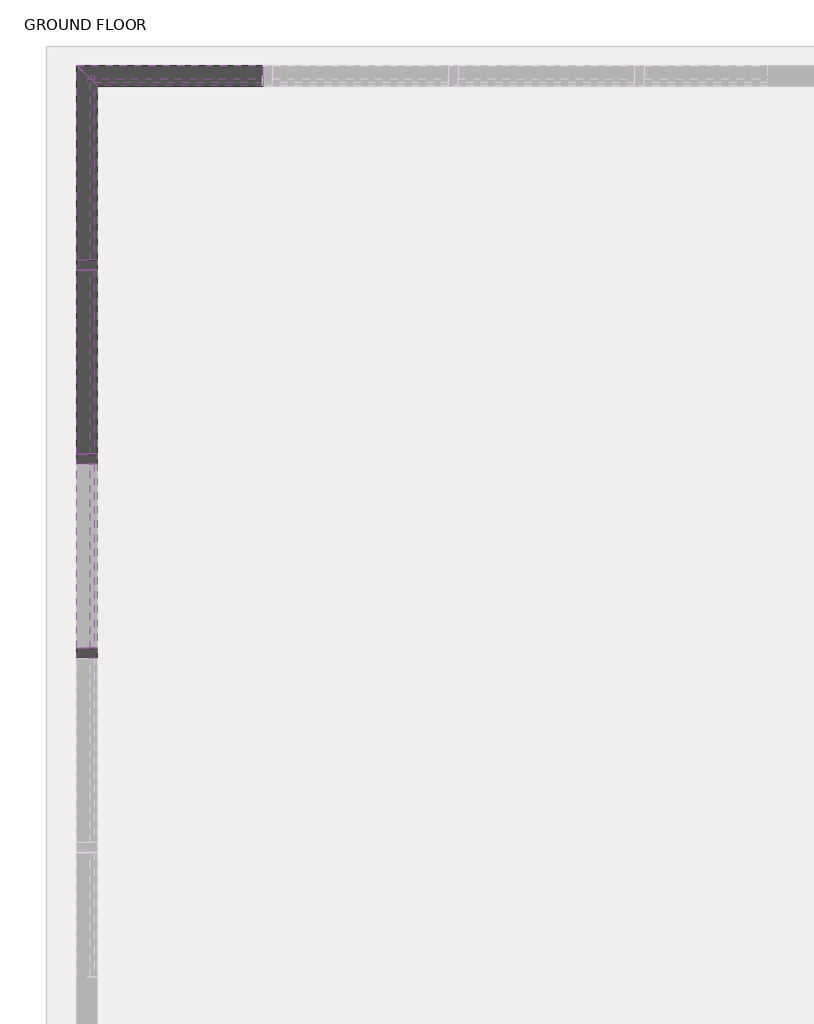
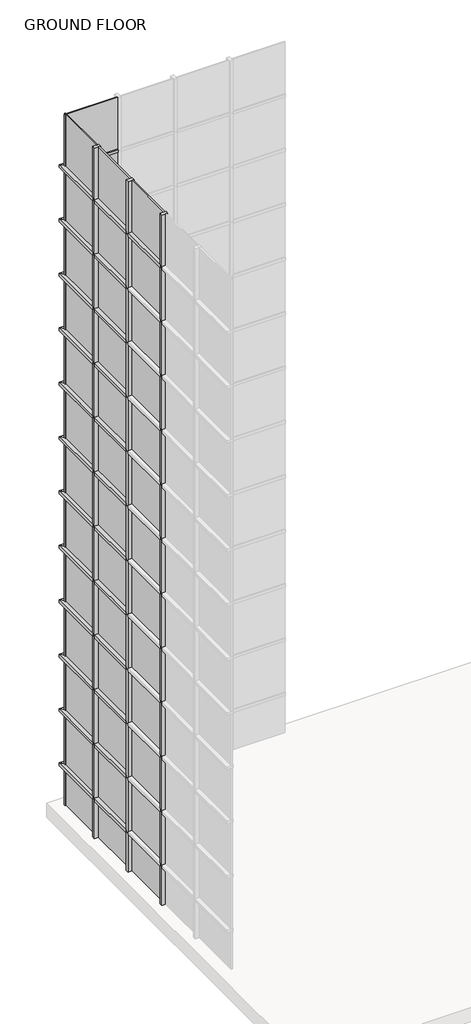
# One storey, part 8 of 16: 76 members, 53 plates.
"""IFC4 building model written with IfcOpenShell, lengths in millimetres."""

from ifc_helpers import new_model, si_unit, origin, place, context, project, spatial, transform, mapped, element, save
from components import member_80100a85, member_b860638c, member_31fee25f, member_49b1bc66, member_a361ce75, system_panel_glazed_5cba32e5, system_panel_glazed_49652e9e

model = new_model("IFC4")

# Units and contexts
model_context = context("Model", 3, world=origin())
ifc_project = project(units=[si_unit("LENGTHUNIT", "METRE", prefix="MILLI")], contexts=[model_context])

# Site, building, storey
site = spatial("IfcSite", under=ifc_project)
building = spatial("IfcBuilding", under=site)
storey = spatial("IfcBuildingStorey", under=building, Name="GROUND FLOOR", Elevation=0.0)

# Members
placement = place(None, origin())
member_shape = member_80100a85(model_context)
element("IfcMember", 1, ObjectType="Rectangular Mullion : 2.5\" x 5\" rectangular", at=placement, inside=storey, context=model_context, shape_type="MappedRepresentation", body=[
    mapped(member_shape, transform((-9124.9017534, 5216.4311965, 1168.8884615), x_axis=(0.0, 0.0, 1.0), y_axis=(-1.0, 0.0, 0.0), z_axis=(0.0, -1.0, 0.0))),
])
element("IfcMember", 2, ObjectType="Rectangular Mullion : 2.5\" x 5\" rectangular", at=placement, inside=storey, context=model_context, shape_type="MappedRepresentation", body=[
    mapped(member_shape, transform((-9124.9017534, 5216.4311965, 2369.5269231), x_axis=(0.0, 0.0, 1.0), y_axis=(-1.0, 0.0, 0.0), z_axis=(0.0, -1.0, 0.0))),
])
element("IfcMember", 3, ObjectType="Rectangular Mullion : 2.5\" x 5\" rectangular", at=placement, inside=storey, context=model_context, shape_type="MappedRepresentation", body=[
    mapped(member_shape, transform((-9124.9017534, 5216.4311965, 3570.1653846), x_axis=(0.0, 0.0, 1.0), y_axis=(-1.0, 0.0, 0.0), z_axis=(0.0, -1.0, 0.0))),
])
element("IfcMember", 4, ObjectType="Rectangular Mullion : 2.5\" x 5\" rectangular", at=placement, inside=storey, context=model_context, shape_type="MappedRepresentation", body=[
    mapped(member_shape, transform((-9124.9017534, 5216.4311965, 4770.8038462), x_axis=(0.0, 0.0, 1.0), y_axis=(-1.0, 0.0, 0.0), z_axis=(0.0, -1.0, 0.0))),
])
element("IfcMember", 5, ObjectType="Rectangular Mullion : 2.5\" x 5\" rectangular", at=placement, inside=storey, context=model_context, shape_type="MappedRepresentation", body=[
    mapped(member_shape, transform((-9124.9017534, 5216.4311965, 5971.4423077), x_axis=(0.0, 0.0, 1.0), y_axis=(-1.0, 0.0, 0.0), z_axis=(0.0, -1.0, 0.0))),
])
element("IfcMember", 6, ObjectType="Rectangular Mullion : 2.5\" x 5\" rectangular", at=placement, inside=storey, context=model_context, shape_type="MappedRepresentation", body=[
    mapped(member_shape, transform((-9124.9017534, 5216.4311965, 7172.0807692), x_axis=(0.0, 0.0, 1.0), y_axis=(-1.0, 0.0, 0.0), z_axis=(0.0, -1.0, 0.0))),
])
element("IfcMember", 7, ObjectType="Rectangular Mullion : 2.5\" x 5\" rectangular", at=placement, inside=storey, context=model_context, shape_type="MappedRepresentation", body=[
    mapped(member_shape, transform((-9124.9017534, 5216.4311965, 8372.7192308), x_axis=(0.0, 0.0, 1.0), y_axis=(-1.0, 0.0, 0.0), z_axis=(0.0, -1.0, 0.0))),
])
element("IfcMember", 8, ObjectType="Rectangular Mullion : 2.5\" x 5\" rectangular", at=placement, inside=storey, context=model_context, shape_type="MappedRepresentation", body=[
    mapped(member_shape, transform((-9124.9017534, 5216.4311965, 9573.3576923), x_axis=(0.0, 0.0, 1.0), y_axis=(-1.0, 0.0, 0.0), z_axis=(0.0, -1.0, 0.0))),
])
element("IfcMember", 9, ObjectType="Rectangular Mullion : 2.5\" x 5\" rectangular", at=placement, inside=storey, context=model_context, shape_type="MappedRepresentation", body=[
    mapped(member_shape, transform((-9124.9017534, 5216.4311965, 10773.9961538), x_axis=(0.0, 0.0, 1.0), y_axis=(-1.0, 0.0, 0.0), z_axis=(0.0, -1.0, 0.0))),
])
element("IfcMember", 10, ObjectType="Rectangular Mullion : 2.5\" x 5\" rectangular", at=placement, inside=storey, context=model_context, shape_type="MappedRepresentation", body=[
    mapped(member_shape, transform((-9124.9017534, 5216.4311965, 11974.6346154), x_axis=(0.0, 0.0, 1.0), y_axis=(-1.0, 0.0, 0.0), z_axis=(0.0, -1.0, 0.0))),
])
element("IfcMember", 11, ObjectType="Rectangular Mullion : 2.5\" x 5\" rectangular", at=placement, inside=storey, context=model_context, shape_type="MappedRepresentation", body=[
    mapped(member_shape, transform((-9124.9017534, 5216.4311965, 13175.2730769), x_axis=(0.0, 0.0, 1.0), y_axis=(-1.0, 0.0, 0.0), z_axis=(0.0, -1.0, 0.0))),
])
element("IfcMember", 12, ObjectType="Rectangular Mullion : 2.5\" x 5\" rectangular", at=placement, inside=storey, context=model_context, shape_type="MappedRepresentation", body=[
    mapped(member_shape, transform((-9124.9017534, 5216.4311965, 14375.9115385), x_axis=(0.0, 0.0, 1.0), y_axis=(-1.0, 0.0, 0.0), z_axis=(0.0, -1.0, 0.0))),
])
member_2_shape = member_b860638c(model_context)
element("IfcMember", 13, ObjectType="Rectangular Mullion : 2.5\" x 5\" rectangular", at=placement, inside=storey, context=model_context, shape_type="MappedRepresentation", body=[
    mapped(member_2_shape, transform((-9124.9017534, 5184.6811965, 0.0), x_axis=(0.0, -1.0, 0.0), y_axis=(-1.0, 0.0, 0.0), z_axis=(0.0, 0.0, -1.0))),
])
element("IfcMember", 14, ObjectType="Rectangular Mullion : 2.5\" x 5\" rectangular", at=placement, inside=storey, context=model_context, shape_type="MappedRepresentation", body=[
    mapped(member_2_shape, transform((-9124.9017534, 3967.3861966, 0.0), x_axis=(0.0, -1.0, 0.0), y_axis=(-1.0, 0.0, 0.0), z_axis=(0.0, 0.0, -1.0))),
])
element("IfcMember", 15, ObjectType="Rectangular Mullion : 2.5\" x 5\" rectangular", at=placement, inside=storey, context=model_context, shape_type="MappedRepresentation", body=[
    mapped(member_2_shape, transform((-9124.9017534, 2750.0911967, 0.0), x_axis=(0.0, -1.0, 0.0), y_axis=(-1.0, 0.0, 0.0), z_axis=(0.0, 0.0, -1.0))),
])
member_3_shape = member_31fee25f(model_context)
element("IfcMember", 16, ObjectType="Rectangular Mullion : 2.5\" x 5\" rectangular", at=placement, inside=storey, context=model_context, shape_type="MappedRepresentation", body=[
    mapped(member_3_shape, transform((-9124.9017534, 5184.6811965, 1168.8884615), x_axis=(0.0, -1.0, 0.0), y_axis=(-1.0, 0.0, 0.0), z_axis=(0.0, 0.0, -1.0))),
])
element("IfcMember", 17, ObjectType="Rectangular Mullion : 2.5\" x 5\" rectangular", at=placement, inside=storey, context=model_context, shape_type="MappedRepresentation", body=[
    mapped(member_3_shape, transform((-9124.9017534, 3967.3861966, 1168.8884615), x_axis=(0.0, -1.0, 0.0), y_axis=(-1.0, 0.0, 0.0), z_axis=(0.0, 0.0, -1.0))),
])
element("IfcMember", 18, ObjectType="Rectangular Mullion : 2.5\" x 5\" rectangular", at=placement, inside=storey, context=model_context, shape_type="MappedRepresentation", body=[
    mapped(member_3_shape, transform((-9124.9017534, 2750.0911967, 1168.8884615), x_axis=(0.0, -1.0, 0.0), y_axis=(-1.0, 0.0, 0.0), z_axis=(0.0, 0.0, -1.0))),
])
element("IfcMember", 19, ObjectType="Rectangular Mullion : 2.5\" x 5\" rectangular", at=placement, inside=storey, context=model_context, shape_type="MappedRepresentation", body=[
    mapped(member_3_shape, transform((-9124.9017534, 5184.6811965, 2369.5269231), x_axis=(0.0, -1.0, 0.0), y_axis=(-1.0, 0.0, 0.0), z_axis=(0.0, 0.0, -1.0))),
])
element("IfcMember", 20, ObjectType="Rectangular Mullion : 2.5\" x 5\" rectangular", at=placement, inside=storey, context=model_context, shape_type="MappedRepresentation", body=[
    mapped(member_3_shape, transform((-9124.9017534, 3967.3861966, 2369.5269231), x_axis=(0.0, -1.0, 0.0), y_axis=(-1.0, 0.0, 0.0), z_axis=(0.0, 0.0, -1.0))),
])
element("IfcMember", 21, ObjectType="Rectangular Mullion : 2.5\" x 5\" rectangular", at=placement, inside=storey, context=model_context, shape_type="MappedRepresentation", body=[
    mapped(member_3_shape, transform((-9124.9017534, 2750.0911967, 2369.5269231), x_axis=(0.0, -1.0, 0.0), y_axis=(-1.0, 0.0, 0.0), z_axis=(0.0, 0.0, -1.0))),
])
element("IfcMember", 22, ObjectType="Rectangular Mullion : 2.5\" x 5\" rectangular", at=placement, inside=storey, context=model_context, shape_type="MappedRepresentation", body=[
    mapped(member_3_shape, transform((-9124.9017534, 5184.6811965, 3570.1653846), x_axis=(0.0, -1.0, 0.0), y_axis=(-1.0, 0.0, 0.0), z_axis=(0.0, 0.0, -1.0))),
])
element("IfcMember", 23, ObjectType="Rectangular Mullion : 2.5\" x 5\" rectangular", at=placement, inside=storey, context=model_context, shape_type="MappedRepresentation", body=[
    mapped(member_3_shape, transform((-9124.9017534, 3967.3861966, 3570.1653846), x_axis=(0.0, -1.0, 0.0), y_axis=(-1.0, 0.0, 0.0), z_axis=(0.0, 0.0, -1.0))),
])
element("IfcMember", 24, ObjectType="Rectangular Mullion : 2.5\" x 5\" rectangular", at=placement, inside=storey, context=model_context, shape_type="MappedRepresentation", body=[
    mapped(member_3_shape, transform((-9124.9017534, 2750.0911967, 3570.1653846), x_axis=(0.0, -1.0, 0.0), y_axis=(-1.0, 0.0, 0.0), z_axis=(0.0, 0.0, -1.0))),
])
element("IfcMember", 25, ObjectType="Rectangular Mullion : 2.5\" x 5\" rectangular", at=placement, inside=storey, context=model_context, shape_type="MappedRepresentation", body=[
    mapped(member_3_shape, transform((-9124.9017534, 5184.6811965, 4770.8038462), x_axis=(0.0, -1.0, 0.0), y_axis=(-1.0, 0.0, 0.0), z_axis=(0.0, 0.0, -1.0))),
])
element("IfcMember", 26, ObjectType="Rectangular Mullion : 2.5\" x 5\" rectangular", at=placement, inside=storey, context=model_context, shape_type="MappedRepresentation", body=[
    mapped(member_3_shape, transform((-9124.9017534, 3967.3861966, 4770.8038462), x_axis=(0.0, -1.0, 0.0), y_axis=(-1.0, 0.0, 0.0), z_axis=(0.0, 0.0, -1.0))),
])
element("IfcMember", 27, ObjectType="Rectangular Mullion : 2.5\" x 5\" rectangular", at=placement, inside=storey, context=model_context, shape_type="MappedRepresentation", body=[
    mapped(member_3_shape, transform((-9124.9017534, 2750.0911967, 4770.8038462), x_axis=(0.0, -1.0, 0.0), y_axis=(-1.0, 0.0, 0.0), z_axis=(0.0, 0.0, -1.0))),
])
element("IfcMember", 28, ObjectType="Rectangular Mullion : 2.5\" x 5\" rectangular", at=placement, inside=storey, context=model_context, shape_type="MappedRepresentation", body=[
    mapped(member_3_shape, transform((-9124.9017534, 5184.6811965, 5971.4423077), x_axis=(0.0, -1.0, 0.0), y_axis=(-1.0, 0.0, 0.0), z_axis=(0.0, 0.0, -1.0))),
])
element("IfcMember", 29, ObjectType="Rectangular Mullion : 2.5\" x 5\" rectangular", at=placement, inside=storey, context=model_context, shape_type="MappedRepresentation", body=[
    mapped(member_3_shape, transform((-9124.9017534, 3967.3861966, 5971.4423077), x_axis=(0.0, -1.0, 0.0), y_axis=(-1.0, 0.0, 0.0), z_axis=(0.0, 0.0, -1.0))),
])
element("IfcMember", 30, ObjectType="Rectangular Mullion : 2.5\" x 5\" rectangular", at=placement, inside=storey, context=model_context, shape_type="MappedRepresentation", body=[
    mapped(member_3_shape, transform((-9124.9017534, 2750.0911967, 5971.4423077), x_axis=(0.0, -1.0, 0.0), y_axis=(-1.0, 0.0, 0.0), z_axis=(0.0, 0.0, -1.0))),
])
element("IfcMember", 31, ObjectType="Rectangular Mullion : 2.5\" x 5\" rectangular", at=placement, inside=storey, context=model_context, shape_type="MappedRepresentation", body=[
    mapped(member_3_shape, transform((-9124.9017534, 5184.6811965, 7172.0807692), x_axis=(0.0, -1.0, 0.0), y_axis=(-1.0, 0.0, 0.0), z_axis=(0.0, 0.0, -1.0))),
])
element("IfcMember", 32, ObjectType="Rectangular Mullion : 2.5\" x 5\" rectangular", at=placement, inside=storey, context=model_context, shape_type="MappedRepresentation", body=[
    mapped(member_3_shape, transform((-9124.9017534, 3967.3861966, 7172.0807692), x_axis=(0.0, -1.0, 0.0), y_axis=(-1.0, 0.0, 0.0), z_axis=(0.0, 0.0, -1.0))),
])
element("IfcMember", 33, ObjectType="Rectangular Mullion : 2.5\" x 5\" rectangular", at=placement, inside=storey, context=model_context, shape_type="MappedRepresentation", body=[
    mapped(member_3_shape, transform((-9124.9017534, 2750.0911967, 7172.0807692), x_axis=(0.0, -1.0, 0.0), y_axis=(-1.0, 0.0, 0.0), z_axis=(0.0, 0.0, -1.0))),
])
element("IfcMember", 34, ObjectType="Rectangular Mullion : 2.5\" x 5\" rectangular", at=placement, inside=storey, context=model_context, shape_type="MappedRepresentation", body=[
    mapped(member_3_shape, transform((-9124.9017534, 5184.6811965, 8372.7192308), x_axis=(0.0, -1.0, 0.0), y_axis=(-1.0, 0.0, 0.0), z_axis=(0.0, 0.0, -1.0))),
])
element("IfcMember", 35, ObjectType="Rectangular Mullion : 2.5\" x 5\" rectangular", at=placement, inside=storey, context=model_context, shape_type="MappedRepresentation", body=[
    mapped(member_3_shape, transform((-9124.9017534, 3967.3861966, 8372.7192308), x_axis=(0.0, -1.0, 0.0), y_axis=(-1.0, 0.0, 0.0), z_axis=(0.0, 0.0, -1.0))),
])
element("IfcMember", 36, ObjectType="Rectangular Mullion : 2.5\" x 5\" rectangular", at=placement, inside=storey, context=model_context, shape_type="MappedRepresentation", body=[
    mapped(member_3_shape, transform((-9124.9017534, 2750.0911967, 8372.7192308), x_axis=(0.0, -1.0, 0.0), y_axis=(-1.0, 0.0, 0.0), z_axis=(0.0, 0.0, -1.0))),
])
element("IfcMember", 37, ObjectType="Rectangular Mullion : 2.5\" x 5\" rectangular", at=placement, inside=storey, context=model_context, shape_type="MappedRepresentation", body=[
    mapped(member_3_shape, transform((-9124.9017534, 5184.6811965, 9573.3576923), x_axis=(0.0, -1.0, 0.0), y_axis=(-1.0, 0.0, 0.0), z_axis=(0.0, 0.0, -1.0))),
])
element("IfcMember", 38, ObjectType="Rectangular Mullion : 2.5\" x 5\" rectangular", at=placement, inside=storey, context=model_context, shape_type="MappedRepresentation", body=[
    mapped(member_3_shape, transform((-9124.9017534, 3967.3861966, 9573.3576923), x_axis=(0.0, -1.0, 0.0), y_axis=(-1.0, 0.0, 0.0), z_axis=(0.0, 0.0, -1.0))),
])
element("IfcMember", 39, ObjectType="Rectangular Mullion : 2.5\" x 5\" rectangular", at=placement, inside=storey, context=model_context, shape_type="MappedRepresentation", body=[
    mapped(member_3_shape, transform((-9124.9017534, 2750.0911967, 9573.3576923), x_axis=(0.0, -1.0, 0.0), y_axis=(-1.0, 0.0, 0.0), z_axis=(0.0, 0.0, -1.0))),
])
element("IfcMember", 40, ObjectType="Rectangular Mullion : 2.5\" x 5\" rectangular", at=placement, inside=storey, context=model_context, shape_type="MappedRepresentation", body=[
    mapped(member_3_shape, transform((-9124.9017534, 5184.6811965, 10773.9961538), x_axis=(0.0, -1.0, 0.0), y_axis=(-1.0, 0.0, 0.0), z_axis=(0.0, 0.0, -1.0))),
])
element("IfcMember", 41, ObjectType="Rectangular Mullion : 2.5\" x 5\" rectangular", at=placement, inside=storey, context=model_context, shape_type="MappedRepresentation", body=[
    mapped(member_3_shape, transform((-9124.9017534, 3967.3861966, 10773.9961538), x_axis=(0.0, -1.0, 0.0), y_axis=(-1.0, 0.0, 0.0), z_axis=(0.0, 0.0, -1.0))),
])
element("IfcMember", 42, ObjectType="Rectangular Mullion : 2.5\" x 5\" rectangular", at=placement, inside=storey, context=model_context, shape_type="MappedRepresentation", body=[
    mapped(member_3_shape, transform((-9124.9017534, 2750.0911967, 10773.9961538), x_axis=(0.0, -1.0, 0.0), y_axis=(-1.0, 0.0, 0.0), z_axis=(0.0, 0.0, -1.0))),
])
element("IfcMember", 43, ObjectType="Rectangular Mullion : 2.5\" x 5\" rectangular", at=placement, inside=storey, context=model_context, shape_type="MappedRepresentation", body=[
    mapped(member_3_shape, transform((-9124.9017534, 5184.6811965, 11974.6346154), x_axis=(0.0, -1.0, 0.0), y_axis=(-1.0, 0.0, 0.0), z_axis=(0.0, 0.0, -1.0))),
])
element("IfcMember", 44, ObjectType="Rectangular Mullion : 2.5\" x 5\" rectangular", at=placement, inside=storey, context=model_context, shape_type="MappedRepresentation", body=[
    mapped(member_3_shape, transform((-9124.9017534, 3967.3861966, 11974.6346154), x_axis=(0.0, -1.0, 0.0), y_axis=(-1.0, 0.0, 0.0), z_axis=(0.0, 0.0, -1.0))),
])
element("IfcMember", 45, ObjectType="Rectangular Mullion : 2.5\" x 5\" rectangular", at=placement, inside=storey, context=model_context, shape_type="MappedRepresentation", body=[
    mapped(member_3_shape, transform((-9124.9017534, 2750.0911967, 11974.6346154), x_axis=(0.0, -1.0, 0.0), y_axis=(-1.0, 0.0, 0.0), z_axis=(0.0, 0.0, -1.0))),
])
element("IfcMember", 46, ObjectType="Rectangular Mullion : 2.5\" x 5\" rectangular", at=placement, inside=storey, context=model_context, shape_type="MappedRepresentation", body=[
    mapped(member_3_shape, transform((-9124.9017534, 5184.6811965, 13175.2730769), x_axis=(0.0, -1.0, 0.0), y_axis=(-1.0, 0.0, 0.0), z_axis=(0.0, 0.0, -1.0))),
])
element("IfcMember", 47, ObjectType="Rectangular Mullion : 2.5\" x 5\" rectangular", at=placement, inside=storey, context=model_context, shape_type="MappedRepresentation", body=[
    mapped(member_3_shape, transform((-9124.9017534, 3967.3861966, 13175.2730769), x_axis=(0.0, -1.0, 0.0), y_axis=(-1.0, 0.0, 0.0), z_axis=(0.0, 0.0, -1.0))),
])
element("IfcMember", 48, ObjectType="Rectangular Mullion : 2.5\" x 5\" rectangular", at=placement, inside=storey, context=model_context, shape_type="MappedRepresentation", body=[
    mapped(member_3_shape, transform((-9124.9017534, 2750.0911967, 13175.2730769), x_axis=(0.0, -1.0, 0.0), y_axis=(-1.0, 0.0, 0.0), z_axis=(0.0, 0.0, -1.0))),
])
element("IfcMember", 49, ObjectType="Rectangular Mullion : 2.5\" x 5\" rectangular", at=placement, inside=storey, context=model_context, shape_type="MappedRepresentation", body=[
    mapped(member_2_shape, transform((-9124.9017534, 5184.6811965, 14375.9115385), x_axis=(0.0, -1.0, 0.0), y_axis=(-1.0, 0.0, 0.0), z_axis=(0.0, 0.0, -1.0))),
])
element("IfcMember", 50, ObjectType="Rectangular Mullion : 2.5\" x 5\" rectangular", at=placement, inside=storey, context=model_context, shape_type="MappedRepresentation", body=[
    mapped(member_2_shape, transform((-9124.9017534, 3967.3861966, 14375.9115385), x_axis=(0.0, -1.0, 0.0), y_axis=(-1.0, 0.0, 0.0), z_axis=(0.0, 0.0, -1.0))),
])
element("IfcMember", 51, ObjectType="Rectangular Mullion : 2.5\" x 5\" rectangular", at=placement, inside=storey, context=model_context, shape_type="MappedRepresentation", body=[
    mapped(member_2_shape, transform((-9124.9017534, 2750.0911967, 14375.9115385), x_axis=(0.0, -1.0, 0.0), y_axis=(-1.0, 0.0, 0.0), z_axis=(0.0, 0.0, -1.0))),
])
member_4_shape = member_49b1bc66(model_context)
element("IfcMember", 52, ObjectType="Rectangular Mullion : 2.5\" x 5\" rectangular", at=placement, inside=storey, context=model_context, shape_type="MappedRepresentation", body=[
    mapped(member_4_shape, transform((-9124.9017534, 3999.1361966, 1168.8884615), x_axis=(0.0, 0.0, 1.0), y_axis=(-1.0, 0.0, 0.0), z_axis=(0.0, -1.0, 0.0))),
])
element("IfcMember", 53, ObjectType="Rectangular Mullion : 2.5\" x 5\" rectangular", at=placement, inside=storey, context=model_context, shape_type="MappedRepresentation", body=[
    mapped(member_4_shape, transform((-9124.9017534, 3999.1361966, 2369.5269231), x_axis=(0.0, 0.0, 1.0), y_axis=(-1.0, 0.0, 0.0), z_axis=(0.0, -1.0, 0.0))),
])
element("IfcMember", 54, ObjectType="Rectangular Mullion : 2.5\" x 5\" rectangular", at=placement, inside=storey, context=model_context, shape_type="MappedRepresentation", body=[
    mapped(member_4_shape, transform((-9124.9017534, 3999.1361966, 3570.1653846), x_axis=(0.0, 0.0, 1.0), y_axis=(-1.0, 0.0, 0.0), z_axis=(0.0, -1.0, 0.0))),
])
element("IfcMember", 55, ObjectType="Rectangular Mullion : 2.5\" x 5\" rectangular", at=placement, inside=storey, context=model_context, shape_type="MappedRepresentation", body=[
    mapped(member_4_shape, transform((-9124.9017534, 3999.1361966, 4770.8038462), x_axis=(0.0, 0.0, 1.0), y_axis=(-1.0, 0.0, 0.0), z_axis=(0.0, -1.0, 0.0))),
])
element("IfcMember", 56, ObjectType="Rectangular Mullion : 2.5\" x 5\" rectangular", at=placement, inside=storey, context=model_context, shape_type="MappedRepresentation", body=[
    mapped(member_4_shape, transform((-9124.9017534, 3999.1361966, 5971.4423077), x_axis=(0.0, 0.0, 1.0), y_axis=(-1.0, 0.0, 0.0), z_axis=(0.0, -1.0, 0.0))),
])
element("IfcMember", 57, ObjectType="Rectangular Mullion : 2.5\" x 5\" rectangular", at=placement, inside=storey, context=model_context, shape_type="MappedRepresentation", body=[
    mapped(member_4_shape, transform((-9124.9017534, 3999.1361966, 7172.0807692), x_axis=(0.0, 0.0, 1.0), y_axis=(-1.0, 0.0, 0.0), z_axis=(0.0, -1.0, 0.0))),
])
element("IfcMember", 58, ObjectType="Rectangular Mullion : 2.5\" x 5\" rectangular", at=placement, inside=storey, context=model_context, shape_type="MappedRepresentation", body=[
    mapped(member_4_shape, transform((-9124.9017534, 3999.1361966, 8372.7192308), x_axis=(0.0, 0.0, 1.0), y_axis=(-1.0, 0.0, 0.0), z_axis=(0.0, -1.0, 0.0))),
])
element("IfcMember", 59, ObjectType="Rectangular Mullion : 2.5\" x 5\" rectangular", at=placement, inside=storey, context=model_context, shape_type="MappedRepresentation", body=[
    mapped(member_4_shape, transform((-9124.9017534, 3999.1361966, 9573.3576923), x_axis=(0.0, 0.0, 1.0), y_axis=(-1.0, 0.0, 0.0), z_axis=(0.0, -1.0, 0.0))),
])
element("IfcMember", 60, ObjectType="Rectangular Mullion : 2.5\" x 5\" rectangular", at=placement, inside=storey, context=model_context, shape_type="MappedRepresentation", body=[
    mapped(member_4_shape, transform((-9124.9017534, 3999.1361966, 10773.9961538), x_axis=(0.0, 0.0, 1.0), y_axis=(-1.0, 0.0, 0.0), z_axis=(0.0, -1.0, 0.0))),
])
element("IfcMember", 61, ObjectType="Rectangular Mullion : 2.5\" x 5\" rectangular", at=placement, inside=storey, context=model_context, shape_type="MappedRepresentation", body=[
    mapped(member_4_shape, transform((-9124.9017534, 3999.1361966, 11974.6346154), x_axis=(0.0, 0.0, 1.0), y_axis=(-1.0, 0.0, 0.0), z_axis=(0.0, -1.0, 0.0))),
])
element("IfcMember", 62, ObjectType="Rectangular Mullion : 2.5\" x 5\" rectangular", at=placement, inside=storey, context=model_context, shape_type="MappedRepresentation", body=[
    mapped(member_4_shape, transform((-9124.9017534, 3999.1361966, 13175.2730769), x_axis=(0.0, 0.0, 1.0), y_axis=(-1.0, 0.0, 0.0), z_axis=(0.0, -1.0, 0.0))),
])
element("IfcMember", 63, ObjectType="Rectangular Mullion : 2.5\" x 5\" rectangular", at=placement, inside=storey, context=model_context, shape_type="MappedRepresentation", body=[
    mapped(member_4_shape, transform((-9124.9017534, 3999.1361966, 14375.9115385), x_axis=(0.0, 0.0, 1.0), y_axis=(-1.0, 0.0, 0.0), z_axis=(0.0, -1.0, 0.0))),
])
element("IfcMember", 64, ObjectType="Rectangular Mullion : 2.5\" x 5\" rectangular", at=placement, inside=storey, context=model_context, shape_type="MappedRepresentation", body=[
    mapped(member_4_shape, transform((-9124.9017534, 2781.8411967, 14375.9115385), x_axis=(0.0, 0.0, 1.0), y_axis=(-1.0, 0.0, 0.0), z_axis=(0.0, -1.0, 0.0))),
])
member_5_shape = member_a361ce75(model_context)
element("IfcMember", 65, ObjectType="Rectangular Mullion : 2.5\" x 5\" rectangular", at=placement, inside=storey, context=model_context, shape_type="MappedRepresentation", body=[
    mapped(member_5_shape, transform((-9124.9017534, 6370.2261968, 1168.8884615), x_axis=(0.0, 0.0, 1.0), y_axis=(0.0, 1.0, 0.0), z_axis=(-1.0, 0.0, 0.0))),
])
element("IfcMember", 66, ObjectType="Rectangular Mullion : 2.5\" x 5\" rectangular", at=placement, inside=storey, context=model_context, shape_type="MappedRepresentation", body=[
    mapped(member_5_shape, transform((-9124.9017534, 6370.2261968, 2369.5269231), x_axis=(0.0, 0.0, 1.0), y_axis=(0.0, 1.0, 0.0), z_axis=(-1.0, 0.0, 0.0))),
])
element("IfcMember", 67, ObjectType="Rectangular Mullion : 2.5\" x 5\" rectangular", at=placement, inside=storey, context=model_context, shape_type="MappedRepresentation", body=[
    mapped(member_5_shape, transform((-9124.9017534, 6370.2261968, 3570.1653846), x_axis=(0.0, 0.0, 1.0), y_axis=(0.0, 1.0, 0.0), z_axis=(-1.0, 0.0, 0.0))),
])
element("IfcMember", 68, ObjectType="Rectangular Mullion : 2.5\" x 5\" rectangular", at=placement, inside=storey, context=model_context, shape_type="MappedRepresentation", body=[
    mapped(member_5_shape, transform((-9124.9017534, 6370.2261968, 4770.8038462), x_axis=(0.0, 0.0, 1.0), y_axis=(0.0, 1.0, 0.0), z_axis=(-1.0, 0.0, 0.0))),
])
element("IfcMember", 69, ObjectType="Rectangular Mullion : 2.5\" x 5\" rectangular", at=placement, inside=storey, context=model_context, shape_type="MappedRepresentation", body=[
    mapped(member_5_shape, transform((-9124.9017534, 6370.2261968, 5971.4423077), x_axis=(0.0, 0.0, 1.0), y_axis=(0.0, 1.0, 0.0), z_axis=(-1.0, 0.0, 0.0))),
])
element("IfcMember", 70, ObjectType="Rectangular Mullion : 2.5\" x 5\" rectangular", at=placement, inside=storey, context=model_context, shape_type="MappedRepresentation", body=[
    mapped(member_5_shape, transform((-9124.9017534, 6370.2261968, 7172.0807692), x_axis=(0.0, 0.0, 1.0), y_axis=(0.0, 1.0, 0.0), z_axis=(-1.0, 0.0, 0.0))),
])
element("IfcMember", 71, ObjectType="Rectangular Mullion : 2.5\" x 5\" rectangular", at=placement, inside=storey, context=model_context, shape_type="MappedRepresentation", body=[
    mapped(member_5_shape, transform((-9124.9017534, 6370.2261968, 8372.7192308), x_axis=(0.0, 0.0, 1.0), y_axis=(0.0, 1.0, 0.0), z_axis=(-1.0, 0.0, 0.0))),
])
element("IfcMember", 72, ObjectType="Rectangular Mullion : 2.5\" x 5\" rectangular", at=placement, inside=storey, context=model_context, shape_type="MappedRepresentation", body=[
    mapped(member_5_shape, transform((-9124.9017534, 6370.2261968, 9573.3576923), x_axis=(0.0, 0.0, 1.0), y_axis=(0.0, 1.0, 0.0), z_axis=(-1.0, 0.0, 0.0))),
])
element("IfcMember", 73, ObjectType="Rectangular Mullion : 2.5\" x 5\" rectangular", at=placement, inside=storey, context=model_context, shape_type="MappedRepresentation", body=[
    mapped(member_5_shape, transform((-9124.9017534, 6370.2261968, 10773.9961538), x_axis=(0.0, 0.0, 1.0), y_axis=(0.0, 1.0, 0.0), z_axis=(-1.0, 0.0, 0.0))),
])
element("IfcMember", 74, ObjectType="Rectangular Mullion : 2.5\" x 5\" rectangular", at=placement, inside=storey, context=model_context, shape_type="MappedRepresentation", body=[
    mapped(member_5_shape, transform((-9124.9017534, 6370.2261968, 11974.6346154), x_axis=(0.0, 0.0, 1.0), y_axis=(0.0, 1.0, 0.0), z_axis=(-1.0, 0.0, 0.0))),
])
element("IfcMember", 75, ObjectType="Rectangular Mullion : 2.5\" x 5\" rectangular", at=placement, inside=storey, context=model_context, shape_type="MappedRepresentation", body=[
    mapped(member_5_shape, transform((-9124.9017534, 6370.2261968, 13175.2730769), x_axis=(0.0, 0.0, 1.0), y_axis=(0.0, 1.0, 0.0), z_axis=(-1.0, 0.0, 0.0))),
])
element("IfcMember", 76, ObjectType="Rectangular Mullion : 2.5\" x 5\" rectangular", at=placement, inside=storey, context=model_context, shape_type="MappedRepresentation", body=[
    mapped(member_5_shape, transform((-9124.9017534, 6370.2261968, 14375.9115385), x_axis=(0.0, 0.0, 1.0), y_axis=(0.0, 1.0, 0.0), z_axis=(-1.0, 0.0, 0.0))),
])

# Plates
system_panel_glazed_shape = system_panel_glazed_5cba32e5(model_context)
element("IfcPlate", 77, ObjectType="System Panel : Glazed", at=placement, inside=storey, context=model_context, shape_type="MappedRepresentation", body=[
    mapped(system_panel_glazed_shape, transform((-7408.447907, 6370.2261968, 0.0), x_axis=(-1.0, 0.0, 0.0), y_axis=(0.0, -1.0, 0.0), z_axis=(0.0, 0.0, 1.0))),
])
element("IfcPlate", 78, ObjectType="System Panel : Glazed", at=placement, inside=storey, context=model_context, shape_type="MappedRepresentation", body=[
    mapped(system_panel_glazed_shape, transform((-8573.9171379, 6370.2261968, 0.0), x_axis=(-1.0, 0.0, 0.0), y_axis=(0.0, -1.0, 0.0), z_axis=(0.0, 0.0, 1.0))),
])
element("IfcPlate", 79, ObjectType="System Panel : Glazed", at=placement, inside=storey, context=model_context, shape_type="MappedRepresentation", body=[
    mapped(system_panel_glazed_shape, transform((-8573.9171379, 6370.2261968, 1200.6384615), x_axis=(-1.0, 0.0, 0.0), y_axis=(0.0, -1.0, 0.0), z_axis=(0.0, 0.0, 1.0))),
])
element("IfcPlate", 80, ObjectType="System Panel : Glazed", at=placement, inside=storey, context=model_context, shape_type="MappedRepresentation", body=[
    mapped(system_panel_glazed_shape, transform((-8573.9171379, 6370.2261968, 2401.2769231), x_axis=(-1.0, 0.0, 0.0), y_axis=(0.0, -1.0, 0.0), z_axis=(0.0, 0.0, 1.0))),
])
element("IfcPlate", 81, ObjectType="System Panel : Glazed", at=placement, inside=storey, context=model_context, shape_type="MappedRepresentation", body=[
    mapped(system_panel_glazed_shape, transform((-8573.9171379, 6370.2261968, 3601.9153846), x_axis=(-1.0, 0.0, 0.0), y_axis=(0.0, -1.0, 0.0), z_axis=(0.0, 0.0, 1.0))),
])
element("IfcPlate", 82, ObjectType="System Panel : Glazed", at=placement, inside=storey, context=model_context, shape_type="MappedRepresentation", body=[
    mapped(system_panel_glazed_shape, transform((-8573.9171379, 6370.2261968, 4802.5538462), x_axis=(-1.0, 0.0, 0.0), y_axis=(0.0, -1.0, 0.0), z_axis=(0.0, 0.0, 1.0))),
])
element("IfcPlate", 83, ObjectType="System Panel : Glazed", at=placement, inside=storey, context=model_context, shape_type="MappedRepresentation", body=[
    mapped(system_panel_glazed_shape, transform((-8573.9171379, 6370.2261968, 6003.1923077), x_axis=(-1.0, 0.0, 0.0), y_axis=(0.0, -1.0, 0.0), z_axis=(0.0, 0.0, 1.0))),
])
element("IfcPlate", 84, ObjectType="System Panel : Glazed", at=placement, inside=storey, context=model_context, shape_type="MappedRepresentation", body=[
    mapped(system_panel_glazed_shape, transform((-8573.9171379, 6370.2261968, 7203.8307692), x_axis=(-1.0, 0.0, 0.0), y_axis=(0.0, -1.0, 0.0), z_axis=(0.0, 0.0, 1.0))),
])
element("IfcPlate", 85, ObjectType="System Panel : Glazed", at=placement, inside=storey, context=model_context, shape_type="MappedRepresentation", body=[
    mapped(system_panel_glazed_shape, transform((-8573.9171379, 6370.2261968, 8404.4692308), x_axis=(-1.0, 0.0, 0.0), y_axis=(0.0, -1.0, 0.0), z_axis=(0.0, 0.0, 1.0))),
])
element("IfcPlate", 86, ObjectType="System Panel : Glazed", at=placement, inside=storey, context=model_context, shape_type="MappedRepresentation", body=[
    mapped(system_panel_glazed_shape, transform((-8573.9171379, 6370.2261968, 9605.1076923), x_axis=(-1.0, 0.0, 0.0), y_axis=(0.0, -1.0, 0.0), z_axis=(0.0, 0.0, 1.0))),
])
element("IfcPlate", 87, ObjectType="System Panel : Glazed", at=placement, inside=storey, context=model_context, shape_type="MappedRepresentation", body=[
    mapped(system_panel_glazed_shape, transform((-8573.9171379, 6370.2261968, 10805.7461538), x_axis=(-1.0, 0.0, 0.0), y_axis=(0.0, -1.0, 0.0), z_axis=(0.0, 0.0, 1.0))),
])
element("IfcPlate", 88, ObjectType="System Panel : Glazed", at=placement, inside=storey, context=model_context, shape_type="MappedRepresentation", body=[
    mapped(system_panel_glazed_shape, transform((-8573.9171379, 6370.2261968, 12006.3846154), x_axis=(-1.0, 0.0, 0.0), y_axis=(0.0, -1.0, 0.0), z_axis=(0.0, 0.0, 1.0))),
])
element("IfcPlate", 89, ObjectType="System Panel : Glazed", at=placement, inside=storey, context=model_context, shape_type="MappedRepresentation", body=[
    mapped(system_panel_glazed_shape, transform((-8573.9171379, 6370.2261968, 13207.0230769), x_axis=(-1.0, 0.0, 0.0), y_axis=(0.0, -1.0, 0.0), z_axis=(0.0, 0.0, 1.0))),
])
element("IfcPlate", 90, ObjectType="System Panel : Glazed", at=placement, inside=storey, context=model_context, shape_type="MappedRepresentation", body=[
    mapped(system_panel_glazed_shape, transform((-8573.9171379, 6370.2261968, 14407.6615385), x_axis=(-1.0, 0.0, 0.0), y_axis=(0.0, -1.0, 0.0), z_axis=(0.0, 0.0, 1.0))),
])
system_panel_glazed_2_shape = system_panel_glazed_49652e9e(model_context)
element("IfcPlate", 91, ObjectType="System Panel : Glazed", at=placement, inside=storey, context=model_context, shape_type="MappedRepresentation", body=[
    mapped(system_panel_glazed_2_shape, transform((-9124.9017534, 5793.3286967, 0.0), x_axis=(0.0, -1.0, 0.0), y_axis=(1.0, 0.0, 0.0), z_axis=(0.0, 0.0, 1.0))),
])
element("IfcPlate", 92, ObjectType="System Panel : Glazed", at=placement, inside=storey, context=model_context, shape_type="MappedRepresentation", body=[
    mapped(system_panel_glazed_2_shape, transform((-9124.9017534, 4576.0336966, 0.0), x_axis=(0.0, -1.0, 0.0), y_axis=(1.0, 0.0, 0.0), z_axis=(0.0, 0.0, 1.0))),
])
element("IfcPlate", 93, ObjectType="System Panel : Glazed", at=placement, inside=storey, context=model_context, shape_type="MappedRepresentation", body=[
    mapped(system_panel_glazed_2_shape, transform((-9124.9017534, 3358.7386966, 0.0), x_axis=(0.0, -1.0, 0.0), y_axis=(1.0, 0.0, 0.0), z_axis=(0.0, 0.0, 1.0))),
])
element("IfcPlate", 94, ObjectType="System Panel : Glazed", at=placement, inside=storey, context=model_context, shape_type="MappedRepresentation", body=[
    mapped(system_panel_glazed_2_shape, transform((-9124.9017534, 5793.3286967, 1200.6384615), x_axis=(0.0, -1.0, 0.0), y_axis=(1.0, 0.0, 0.0), z_axis=(0.0, 0.0, 1.0))),
])
element("IfcPlate", 95, ObjectType="System Panel : Glazed", at=placement, inside=storey, context=model_context, shape_type="MappedRepresentation", body=[
    mapped(system_panel_glazed_2_shape, transform((-9124.9017534, 4576.0336966, 1200.6384615), x_axis=(0.0, -1.0, 0.0), y_axis=(1.0, 0.0, 0.0), z_axis=(0.0, 0.0, 1.0))),
])
element("IfcPlate", 96, ObjectType="System Panel : Glazed", at=placement, inside=storey, context=model_context, shape_type="MappedRepresentation", body=[
    mapped(system_panel_glazed_2_shape, transform((-9124.9017534, 3358.7386966, 1200.6384615), x_axis=(0.0, -1.0, 0.0), y_axis=(1.0, 0.0, 0.0), z_axis=(0.0, 0.0, 1.0))),
])
element("IfcPlate", 97, ObjectType="System Panel : Glazed", at=placement, inside=storey, context=model_context, shape_type="MappedRepresentation", body=[
    mapped(system_panel_glazed_2_shape, transform((-9124.9017534, 5793.3286967, 2401.2769231), x_axis=(0.0, -1.0, 0.0), y_axis=(1.0, 0.0, 0.0), z_axis=(0.0, 0.0, 1.0))),
])
element("IfcPlate", 98, ObjectType="System Panel : Glazed", at=placement, inside=storey, context=model_context, shape_type="MappedRepresentation", body=[
    mapped(system_panel_glazed_2_shape, transform((-9124.9017534, 4576.0336966, 2401.2769231), x_axis=(0.0, -1.0, 0.0), y_axis=(1.0, 0.0, 0.0), z_axis=(0.0, 0.0, 1.0))),
])
element("IfcPlate", 99, ObjectType="System Panel : Glazed", at=placement, inside=storey, context=model_context, shape_type="MappedRepresentation", body=[
    mapped(system_panel_glazed_2_shape, transform((-9124.9017534, 3358.7386966, 2401.2769231), x_axis=(0.0, -1.0, 0.0), y_axis=(1.0, 0.0, 0.0), z_axis=(0.0, 0.0, 1.0))),
])
element("IfcPlate", 100, ObjectType="System Panel : Glazed", at=placement, inside=storey, context=model_context, shape_type="MappedRepresentation", body=[
    mapped(system_panel_glazed_2_shape, transform((-9124.9017534, 5793.3286967, 3601.9153846), x_axis=(0.0, -1.0, 0.0), y_axis=(1.0, 0.0, 0.0), z_axis=(0.0, 0.0, 1.0))),
])
element("IfcPlate", 101, ObjectType="System Panel : Glazed", at=placement, inside=storey, context=model_context, shape_type="MappedRepresentation", body=[
    mapped(system_panel_glazed_2_shape, transform((-9124.9017534, 4576.0336966, 3601.9153846), x_axis=(0.0, -1.0, 0.0), y_axis=(1.0, 0.0, 0.0), z_axis=(0.0, 0.0, 1.0))),
])
element("IfcPlate", 102, ObjectType="System Panel : Glazed", at=placement, inside=storey, context=model_context, shape_type="MappedRepresentation", body=[
    mapped(system_panel_glazed_2_shape, transform((-9124.9017534, 3358.7386966, 3601.9153846), x_axis=(0.0, -1.0, 0.0), y_axis=(1.0, 0.0, 0.0), z_axis=(0.0, 0.0, 1.0))),
])
element("IfcPlate", 103, ObjectType="System Panel : Glazed", at=placement, inside=storey, context=model_context, shape_type="MappedRepresentation", body=[
    mapped(system_panel_glazed_2_shape, transform((-9124.9017534, 5793.3286967, 4802.5538462), x_axis=(0.0, -1.0, 0.0), y_axis=(1.0, 0.0, 0.0), z_axis=(0.0, 0.0, 1.0))),
])
element("IfcPlate", 104, ObjectType="System Panel : Glazed", at=placement, inside=storey, context=model_context, shape_type="MappedRepresentation", body=[
    mapped(system_panel_glazed_2_shape, transform((-9124.9017534, 4576.0336966, 4802.5538462), x_axis=(0.0, -1.0, 0.0), y_axis=(1.0, 0.0, 0.0), z_axis=(0.0, 0.0, 1.0))),
])
element("IfcPlate", 105, ObjectType="System Panel : Glazed", at=placement, inside=storey, context=model_context, shape_type="MappedRepresentation", body=[
    mapped(system_panel_glazed_2_shape, transform((-9124.9017534, 3358.7386966, 4802.5538462), x_axis=(0.0, -1.0, 0.0), y_axis=(1.0, 0.0, 0.0), z_axis=(0.0, 0.0, 1.0))),
])
element("IfcPlate", 106, ObjectType="System Panel : Glazed", at=placement, inside=storey, context=model_context, shape_type="MappedRepresentation", body=[
    mapped(system_panel_glazed_2_shape, transform((-9124.9017534, 5793.3286967, 6003.1923077), x_axis=(0.0, -1.0, 0.0), y_axis=(1.0, 0.0, 0.0), z_axis=(0.0, 0.0, 1.0))),
])
element("IfcPlate", 107, ObjectType="System Panel : Glazed", at=placement, inside=storey, context=model_context, shape_type="MappedRepresentation", body=[
    mapped(system_panel_glazed_2_shape, transform((-9124.9017534, 4576.0336966, 6003.1923077), x_axis=(0.0, -1.0, 0.0), y_axis=(1.0, 0.0, 0.0), z_axis=(0.0, 0.0, 1.0))),
])
element("IfcPlate", 108, ObjectType="System Panel : Glazed", at=placement, inside=storey, context=model_context, shape_type="MappedRepresentation", body=[
    mapped(system_panel_glazed_2_shape, transform((-9124.9017534, 3358.7386966, 6003.1923077), x_axis=(0.0, -1.0, 0.0), y_axis=(1.0, 0.0, 0.0), z_axis=(0.0, 0.0, 1.0))),
])
element("IfcPlate", 109, ObjectType="System Panel : Glazed", at=placement, inside=storey, context=model_context, shape_type="MappedRepresentation", body=[
    mapped(system_panel_glazed_2_shape, transform((-9124.9017534, 5793.3286967, 7203.8307692), x_axis=(0.0, -1.0, 0.0), y_axis=(1.0, 0.0, 0.0), z_axis=(0.0, 0.0, 1.0))),
])
element("IfcPlate", 110, ObjectType="System Panel : Glazed", at=placement, inside=storey, context=model_context, shape_type="MappedRepresentation", body=[
    mapped(system_panel_glazed_2_shape, transform((-9124.9017534, 4576.0336966, 7203.8307692), x_axis=(0.0, -1.0, 0.0), y_axis=(1.0, 0.0, 0.0), z_axis=(0.0, 0.0, 1.0))),
])
element("IfcPlate", 111, ObjectType="System Panel : Glazed", at=placement, inside=storey, context=model_context, shape_type="MappedRepresentation", body=[
    mapped(system_panel_glazed_2_shape, transform((-9124.9017534, 3358.7386966, 7203.8307692), x_axis=(0.0, -1.0, 0.0), y_axis=(1.0, 0.0, 0.0), z_axis=(0.0, 0.0, 1.0))),
])
element("IfcPlate", 112, ObjectType="System Panel : Glazed", at=placement, inside=storey, context=model_context, shape_type="MappedRepresentation", body=[
    mapped(system_panel_glazed_2_shape, transform((-9124.9017534, 5793.3286967, 8404.4692308), x_axis=(0.0, -1.0, 0.0), y_axis=(1.0, 0.0, 0.0), z_axis=(0.0, 0.0, 1.0))),
])
element("IfcPlate", 113, ObjectType="System Panel : Glazed", at=placement, inside=storey, context=model_context, shape_type="MappedRepresentation", body=[
    mapped(system_panel_glazed_2_shape, transform((-9124.9017534, 4576.0336966, 8404.4692308), x_axis=(0.0, -1.0, 0.0), y_axis=(1.0, 0.0, 0.0), z_axis=(0.0, 0.0, 1.0))),
])
element("IfcPlate", 114, ObjectType="System Panel : Glazed", at=placement, inside=storey, context=model_context, shape_type="MappedRepresentation", body=[
    mapped(system_panel_glazed_2_shape, transform((-9124.9017534, 3358.7386966, 8404.4692308), x_axis=(0.0, -1.0, 0.0), y_axis=(1.0, 0.0, 0.0), z_axis=(0.0, 0.0, 1.0))),
])
element("IfcPlate", 115, ObjectType="System Panel : Glazed", at=placement, inside=storey, context=model_context, shape_type="MappedRepresentation", body=[
    mapped(system_panel_glazed_2_shape, transform((-9124.9017534, 5793.3286967, 9605.1076923), x_axis=(0.0, -1.0, 0.0), y_axis=(1.0, 0.0, 0.0), z_axis=(0.0, 0.0, 1.0))),
])
element("IfcPlate", 116, ObjectType="System Panel : Glazed", at=placement, inside=storey, context=model_context, shape_type="MappedRepresentation", body=[
    mapped(system_panel_glazed_2_shape, transform((-9124.9017534, 4576.0336966, 9605.1076923), x_axis=(0.0, -1.0, 0.0), y_axis=(1.0, 0.0, 0.0), z_axis=(0.0, 0.0, 1.0))),
])
element("IfcPlate", 117, ObjectType="System Panel : Glazed", at=placement, inside=storey, context=model_context, shape_type="MappedRepresentation", body=[
    mapped(system_panel_glazed_2_shape, transform((-9124.9017534, 3358.7386966, 9605.1076923), x_axis=(0.0, -1.0, 0.0), y_axis=(1.0, 0.0, 0.0), z_axis=(0.0, 0.0, 1.0))),
])
element("IfcPlate", 118, ObjectType="System Panel : Glazed", at=placement, inside=storey, context=model_context, shape_type="MappedRepresentation", body=[
    mapped(system_panel_glazed_2_shape, transform((-9124.9017534, 5793.3286967, 10805.7461538), x_axis=(0.0, -1.0, 0.0), y_axis=(1.0, 0.0, 0.0), z_axis=(0.0, 0.0, 1.0))),
])
element("IfcPlate", 119, ObjectType="System Panel : Glazed", at=placement, inside=storey, context=model_context, shape_type="MappedRepresentation", body=[
    mapped(system_panel_glazed_2_shape, transform((-9124.9017534, 4576.0336966, 10805.7461538), x_axis=(0.0, -1.0, 0.0), y_axis=(1.0, 0.0, 0.0), z_axis=(0.0, 0.0, 1.0))),
])
element("IfcPlate", 120, ObjectType="System Panel : Glazed", at=placement, inside=storey, context=model_context, shape_type="MappedRepresentation", body=[
    mapped(system_panel_glazed_2_shape, transform((-9124.9017534, 3358.7386966, 10805.7461538), x_axis=(0.0, -1.0, 0.0), y_axis=(1.0, 0.0, 0.0), z_axis=(0.0, 0.0, 1.0))),
])
element("IfcPlate", 121, ObjectType="System Panel : Glazed", at=placement, inside=storey, context=model_context, shape_type="MappedRepresentation", body=[
    mapped(system_panel_glazed_2_shape, transform((-9124.9017534, 5793.3286967, 12006.3846154), x_axis=(0.0, -1.0, 0.0), y_axis=(1.0, 0.0, 0.0), z_axis=(0.0, 0.0, 1.0))),
])
element("IfcPlate", 122, ObjectType="System Panel : Glazed", at=placement, inside=storey, context=model_context, shape_type="MappedRepresentation", body=[
    mapped(system_panel_glazed_2_shape, transform((-9124.9017534, 4576.0336966, 12006.3846154), x_axis=(0.0, -1.0, 0.0), y_axis=(1.0, 0.0, 0.0), z_axis=(0.0, 0.0, 1.0))),
])
element("IfcPlate", 123, ObjectType="System Panel : Glazed", at=placement, inside=storey, context=model_context, shape_type="MappedRepresentation", body=[
    mapped(system_panel_glazed_2_shape, transform((-9124.9017534, 3358.7386966, 12006.3846154), x_axis=(0.0, -1.0, 0.0), y_axis=(1.0, 0.0, 0.0), z_axis=(0.0, 0.0, 1.0))),
])
element("IfcPlate", 124, ObjectType="System Panel : Glazed", at=placement, inside=storey, context=model_context, shape_type="MappedRepresentation", body=[
    mapped(system_panel_glazed_2_shape, transform((-9124.9017534, 5793.3286967, 13207.0230769), x_axis=(0.0, -1.0, 0.0), y_axis=(1.0, 0.0, 0.0), z_axis=(0.0, 0.0, 1.0))),
])
element("IfcPlate", 125, ObjectType="System Panel : Glazed", at=placement, inside=storey, context=model_context, shape_type="MappedRepresentation", body=[
    mapped(system_panel_glazed_2_shape, transform((-9124.9017534, 4576.0336966, 13207.0230769), x_axis=(0.0, -1.0, 0.0), y_axis=(1.0, 0.0, 0.0), z_axis=(0.0, 0.0, 1.0))),
])
element("IfcPlate", 126, ObjectType="System Panel : Glazed", at=placement, inside=storey, context=model_context, shape_type="MappedRepresentation", body=[
    mapped(system_panel_glazed_2_shape, transform((-9124.9017534, 3358.7386966, 13207.0230769), x_axis=(0.0, -1.0, 0.0), y_axis=(1.0, 0.0, 0.0), z_axis=(0.0, 0.0, 1.0))),
])
element("IfcPlate", 127, ObjectType="System Panel : Glazed", at=placement, inside=storey, context=model_context, shape_type="MappedRepresentation", body=[
    mapped(system_panel_glazed_2_shape, transform((-9124.9017534, 5793.3286967, 14407.6615385), x_axis=(0.0, -1.0, 0.0), y_axis=(1.0, 0.0, 0.0), z_axis=(0.0, 0.0, 1.0))),
])
element("IfcPlate", 128, ObjectType="System Panel : Glazed", at=placement, inside=storey, context=model_context, shape_type="MappedRepresentation", body=[
    mapped(system_panel_glazed_2_shape, transform((-9124.9017534, 4576.0336966, 14407.6615385), x_axis=(0.0, -1.0, 0.0), y_axis=(1.0, 0.0, 0.0), z_axis=(0.0, 0.0, 1.0))),
])
element("IfcPlate", 129, ObjectType="System Panel : Glazed", at=placement, inside=storey, context=model_context, shape_type="MappedRepresentation", body=[
    mapped(system_panel_glazed_2_shape, transform((-9124.9017534, 3358.7386966, 14407.6615385), x_axis=(0.0, -1.0, 0.0), y_axis=(1.0, 0.0, 0.0), z_axis=(0.0, 0.0, 1.0))),
])

save(model, "model.ifc")

# Revit data of these elements
# Type "Rectangular Mullion : 2.5\" x 5\" rectangular"
#   built-in parameter 1007304 = 0.416667 (stored number, unit not read)
#   built-in parameter 1007301 = 0.104167 (stored number, unit not read)
#   built-in parameter 1007300 = 0.104167 (stored number, unit not read)
# Type "System Panel : Glazed"
#   Construction Type Id = "GSP4R"
#   Analytic Construction = "1/8 in Pilkington single glazing"
#   Visual Light Transmittance = 0.9
#   Solar Heat Gain Coefficient = 0.86
#   Heat Transfer Coefficient (U) = 1.18115 BTU/(h·ft²·°F)
#   Define Thermal Properties by = 1
# Elements 1, 2, 3, 4, 5, 6, 7, 8, 9, 10, 11, 12, 13, 14, 15, 16, 17, 18, 19, 20, 21, 22, 23, 24, 25, 26, 27, 28, 29, 30, 31, 32, 33, 34, 35, 36, 37, 38, 39, 40, 41, 42, 43, 44, 45, 46, 47, 48, 49, 50, 51, 52, 53, 54, 55, 56, 57, 58, 59, 60, 61, 62, 63, 64, 65, 66, 67, 68, 69, 70, 71, 72, 73, 74, 75, 76 (IfcMember, "Rectangular Mullion : 2.5\" x 5\" rectangular")
#   Phase Created = New Construction
#   Materials on its faces: "Aluminum"
# Elements 77, 78, 79, 80, 81, 82, 83, 84, 85, 86, 87, 88, 89, 90, 91, 92, 93, 94, 95, 96, 97, 98, 99, 100, 101, 102, 103, 104, 105, 106, 107, 108, 109, 110, 111, 112, 113, 114, 115, 116, 117, 118, 119, 120, 121, 122, 123, 124, 125, 126, 127, 128, 129 (IfcPlate, "System Panel : Glazed")
#   Phase Created = New Construction
#   Materials on its faces: "Glass"
# Materials
#   "Aluminum": class "Metal", colour RGB 247 247 247, transparency 0, Description = "Aluminum 6061", Cost = 0
#   "Glass": class "Glass", colour RGB 0 128 192, transparency 0.75, Description = "Soda Lime Glass", Cost = 0
